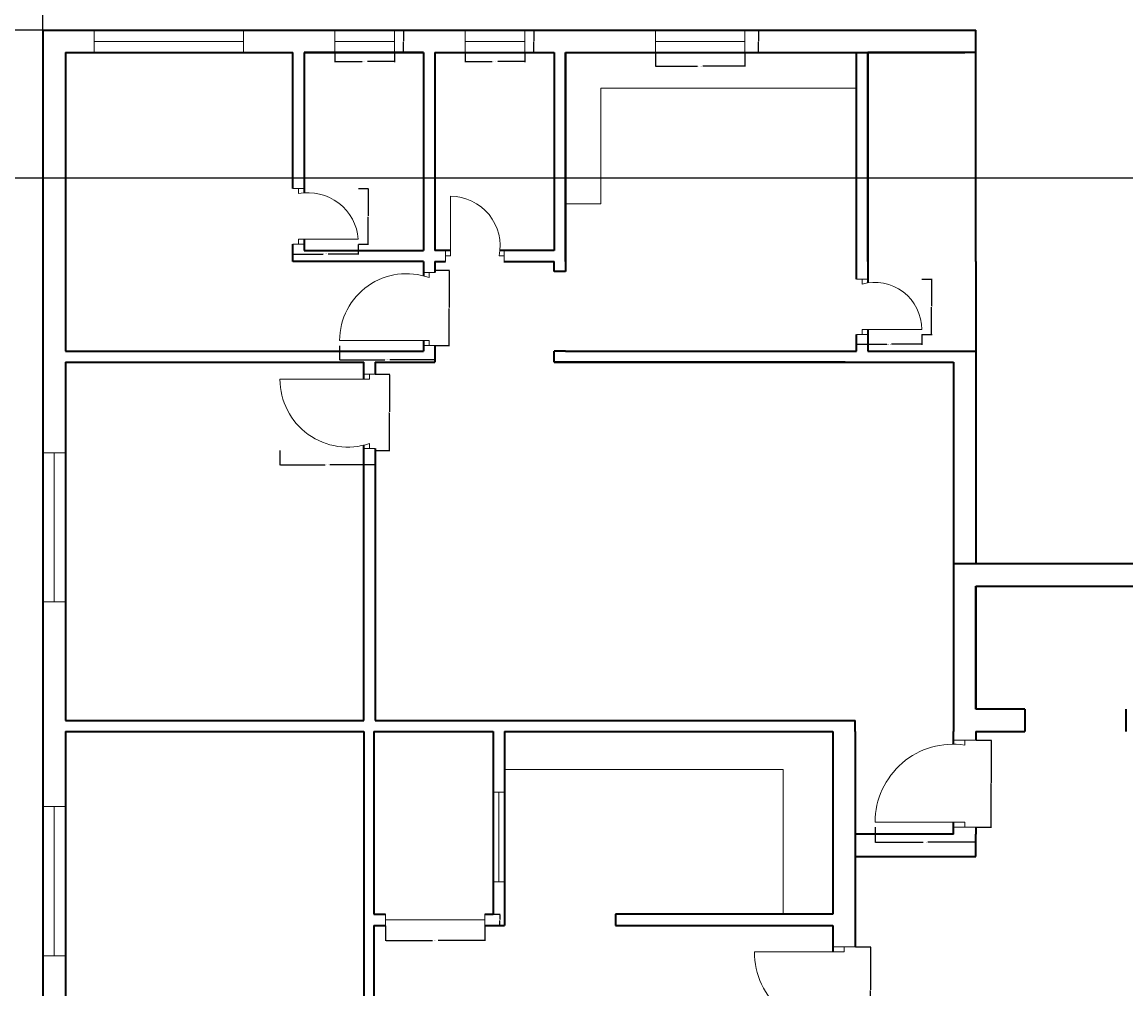
# Model space of a CAD drawing. Units: inches. Extents: x 2120 to 4013, y 1390 to 3019.
# Tile 52 of 59: x 3063 to 3507, y 1967 to 2356. Entities that reach past the tile are written whole.
import ezdxf

# ---------------------------------------------------------------- set-up
doc = ezdxf.new("R2010")
doc.units = ezdxf.units.IN
for name, color, linetype, lineweight in [('A-ANNO-DIMS', 2, 'Continuous', 18), ('A-ANNO-SYMB', 2, 'Continuous', 25), ('A-DOOR', 3, 'Continuous', 18), ('A-FLOR-CASE', 8, 'Continuous', 18), ('A-FURN', 8, 'Continuous', 13), ('A-GLAZ', 4, 'Continuous', 18), ('A-WALL', 7, 'Continuous', 35)]:
    doc.layers.add(name, color=color, linetype=linetype, lineweight=lineweight)
doc.styles.get("Standard").update_dxf_attribs({"font": 'arial.ttf'})
doc.dimstyles.get("Standard").update_dxf_attribs({"dimtxt": 0.18, "dimasz": 0.18, "dimexe": 0.18, "dimexo": 0.0625, "dimgap": 0.09, "dimtad": 0, "dimtih": 1, "dimtoh": 1, "dimdec": 4, "dimzin": 0, "dimdsep": 46, "dimtxsty": 'Standard', "dimcen": 0.09, "dimadec": 0, "dimazin": 0, "dimtfac": 1, "dimtdec": 4, "dimtofl": 0, "dimtmove": 0, "dimatfit": 3, "dimfxl": 1, "dimtolj": 1, "dimtzin": 0, "dimarcsym": 0})

# ---------------------------------------------------------------- blocks, each defined once
blk = doc.blocks.new('DOOR-SWING-24IN-96p73DEG')
for p, q in [((4.5, 22.36), (0, 22.36)), ((0, 22.36), (2.25, 22.36)), ((2.25, 22.36), (2.25, 20.36)), ((2.25, 0), (2.25, 2)), ((2.25, 2), (26.25, 2)), ((4.5, 0), (0, 0)), ((0, 0), (2.25, 0))]:
    blk.add_line(p, q)
blk.add_arc((6.09, 0.51), 20.22, 4.2154, 100.9483)
blk = doc.blocks.new('DOOR-SWING-24IN-101p88DEG')
for p, q in [((2, 2.25), (2, 26.25)), ((0, 4.5), (0, 0)), ((23.48, 4.5), (23.48, 0)), ((0, 0), (0, 2.25)), ((0, 2.25), (2, 2.25)), ((23.48, 2.25), (21.48, 2.25)), ((23.48, 0), (23.48, 2.25))]:
    blk.add_line(p, q)
blk.add_arc((2, 6.35), 19.9, 348.1217, 90)
blk = doc.blocks.new('DOOR-SWING-24IN-105p37DEG')
for p, q in [((4.5, 22.29), (0, 22.29)), ((0, 22.29), (2.25, 22.29)), ((2.25, 22.29), (2.25, 20.29)), ((0, 0), (4.5, 0)), ((2.25, 0), (2.25, 2)), ((2.25, 2), (26.25, 2)), ((4.5, 0), (2.25, 0))]:
    blk.add_line(p, q)
blk.add_arc((7.28, 2), 18.97, 0, 105.3718)
blk = doc.blocks.new('DOOR-SWING-36IN-109p78DEG')
for p, q in [((33.75, 29.31), (38.25, 29.31)), ((38.25, 29.31), (36, 29.31)), ((36, 29.31), (36, 27.31)), ((36, 2), (0, 2)), ((33.75, 0), (38.25, 0)), ((38.25, 0), (35.24, 0)), ((35.24, 0), (36, 0)), ((36, 0), (36, 2))]:
    blk.add_line(p, q)
blk.add_arc((26.9, 2), 26.9, 70.2228, 180)
blk = doc.blocks.new('DOOR-SWING-36IN-108p68DEG')
for p, q in [((36, 27.83), (0, 27.83)), ((38.25, 29.83), (33.75, 29.83)), ((33.75, 29.83), (36, 29.83)), ((36, 29.83), (36, 27.83)), ((36, 0), (36, 2)), ((33.75, 0), (38.25, 0)), ((38.25, 0), (36, 0))]:
    blk.add_line(p, q)
blk.add_arc((27.27, 27.83), 27.27, 180, 288.6764)
blk = doc.blocks.new('DOOR-SWING-36IN-98p95DEG')
for p, q in [((36, 32.77), (0, 32.77)), ((31.5, 34.77), (40.5, 34.77)), ((40.5, 34.77), (36, 34.77)), ((36, 34.77), (36, 32.77)), ((31.5, 0), (40.5, 0)), ((36, 0), (36, 2)), ((40.5, 0), (36, 0))]:
    blk.add_line(p, q)
blk.add_arc((31.15, 32.77), 31.15, 180, 278.9496)
blk = doc.blocks.new('DOOR-SWING-36IN-98p61DEG')
for p, q in [((40.5, 34.96), (31.5, 34.96)), ((31.5, 34.96), (36, 34.96)), ((36, 34.96), (36, 32.96)), ((36, 2), (0, 2)), ((31.5, 0), (40.5, 0)), ((36, 0), (36, 2)), ((40.5, 0), (36, 0))]:
    blk.add_line(p, q)
blk.add_arc((31.31, 2), 31.31, 81.386, 180)
blk = doc.blocks.new('WIN-PLAN-24IN')
for p, q in [((0, 0), (0, 9)), ((0, 9), (0, 4.5)), ((24, 4.5), (24, 9)), ((24, 9), (24, 0)), ((0, 4.5), (24, 4.5)), ((0, 0), (0, 0))]:
    blk.add_line(p, q)
blk = doc.blocks.new('WIN-PLAN-24IN-02')
for p, q in [((0, 0), (0, 9)), ((0, 9), (0, 4.5)), ((24, 4.5), (24, 9)), ((24, 9), (24, 0)), ((0, 4.5), (24, 4.5))]:
    blk.add_line(p, q)
blk = doc.blocks.new('WIN-PLAN-60IN')
for p, q in [((0, 9), (0, 0)), ((60, 4.5), (60, 9)), ((60, 9), (60, 0)), ((0, 0), (0, 4.5)), ((0, 4.5), (60, 4.5))]:
    blk.add_line(p, q)
blk = doc.blocks.new('WIN-PLAN-60IN-02')
for p, q in [((0, 0), (0, 9)), ((0, 9), (0, 4.5)), ((60, 4.5), (60, 9)), ((60, 9), (60, 0)), ((0, 4.5), (60, 4.5))]:
    blk.add_line(p, q)
blk = doc.blocks.new('WIN-PLAN-36IN')
for p, q in [((0, 0), (0, 9)), ((0, 9), (0, 4.5)), ((36, 4.5), (36, 9)), ((36, 9), (36, 0)), ((0, 4.5), (36, 4.5))]:
    blk.add_line(p, q)
blk = doc.blocks.new('WIN-PLAN-36IN-02')
for p, q in [((2.25, 36), (0, 36)), ((0, 36), (4.5, 36)), ((2.25, 0), (2.25, 36)), ((0, 0), (4.5, 0)), ((4.5, 0), (2.25, 0))]:
    blk.add_line(p, q)
blk = doc.blocks.new('WIN-PLAN-40IN')
for p, q in [((0, 4.5), (0, 0)), ((39.95, 4.5), (39.95, 0)), ((39.95, 2.25), (0, 2.25)), ((39.95, 0), (39.95, 2.25))]:
    blk.add_line(p, q)
blk = doc.blocks.new('*D113')
at = {"layer": 'A-ANNO-DIMS', "color": 0, "lineweight": -2, "transparency": 16777216}
for p, q in [((3172.23, 2266.43), (3172.23, 2262.37)), ((3198.48, 2266.43), (3198.48, 2262.37)), ((3172.41, 2262.55), (3184.37, 2262.55)), ((3198.3, 2262.55), (3186.35, 2262.55))]:
    blk.add_line(p, q, dxfattribs=at)
at = {"layer": 'A-ANNO-DIMS', "color": 0, "transparency": 16777216}
for points in [[(3172.41, 2262.58), (3172.41, 2262.52), (3172.23, 2262.55)], [(3198.3, 2262.58), (3198.3, 2262.52), (3198.48, 2262.55)]]:
    blk.add_solid(points, dxfattribs=at)
at = {"layer": 'Defpoints', "color": 0, "transparency": 16777216}
for p in [(3172.23, 2266.49), (3198.48, 2266.49), (3198.48, 2262.55)]:
    blk.add_point(p, dxfattribs=at)
at = {"layer": 'A-ANNO-DIMS', "color": 0, "transparency": 16777216, "insert": (3185.36, 2262.55), "char_height": 0.18, "attachment_point": 5}
blk.add_mtext('\\A1;SWING 26 TYP.', dxfattribs=at)
blk = doc.blocks.new('*D114')
at = {"layer": 'A-ANNO-DIMS', "color": 0, "lineweight": -2, "transparency": 16777216}
for p, q in [((3198.55, 2288.85), (3202.6, 2288.85)), ((3202.42, 2288.67), (3202.42, 2277.85)), ((3202.42, 2266.67), (3202.42, 2277.49)), ((3198.55, 2266.49), (3202.6, 2266.49))]:
    blk.add_line(p, q, dxfattribs=at)
at = {"layer": 'A-ANNO-DIMS', "color": 0, "transparency": 16777216}
for points in [[(3202.39, 2288.67), (3202.45, 2288.67), (3202.42, 2288.85)], [(3202.39, 2266.67), (3202.45, 2266.67), (3202.42, 2266.49)]]:
    blk.add_solid(points, dxfattribs=at)
at = {"layer": 'Defpoints', "color": 0, "transparency": 16777216}
for p in [(3198.48, 2288.85), (3202.42, 2288.85), (3198.48, 2266.49)]:
    blk.add_point(p, dxfattribs=at)
at = {"layer": 'A-ANNO-DIMS', "color": 0, "transparency": 16777216, "insert": (3202.42, 2277.67), "char_height": 0.18, "attachment_point": 5}
blk.add_mtext('\\A1;22 TYP.', dxfattribs=at)
blk = doc.blocks.new('*D117')
at = {"layer": 'A-ANNO-DIMS', "color": 0, "lineweight": -2, "transparency": 16777216}
for p, q in [((3398.73, 2230.14), (3398.73, 2226.08)), ((3424.98, 2230.14), (3424.98, 2226.08)), ((3398.91, 2226.26), (3410.87, 2226.26)), ((3424.8, 2226.26), (3412.85, 2226.26))]:
    blk.add_line(p, q, dxfattribs=at)
at = {"layer": 'A-ANNO-DIMS', "color": 0, "transparency": 16777216}
for points in [[(3398.91, 2226.29), (3398.91, 2226.23), (3398.73, 2226.26)], [(3424.8, 2226.29), (3424.8, 2226.23), (3424.98, 2226.26)]]:
    blk.add_solid(points, dxfattribs=at)
at = {"layer": 'Defpoints', "color": 0, "transparency": 16777216}
for p in [(3398.73, 2230.2), (3424.98, 2230.2), (3424.98, 2226.26)]:
    blk.add_point(p, dxfattribs=at)
at = {"layer": 'A-ANNO-DIMS', "color": 0, "transparency": 16777216, "insert": (3411.86, 2226.26), "char_height": 0.18, "attachment_point": 5}
blk.add_mtext('\\A1;SWING 26 TYP.', dxfattribs=at)
blk = doc.blocks.new('*D118')
at = {"layer": 'A-ANNO-DIMS', "color": 0, "lineweight": -2, "transparency": 16777216}
for p, q in [((3425.05, 2252.49), (3429.1, 2252.49)), ((3428.92, 2252.31), (3428.92, 2241.53)), ((3428.92, 2230.38), (3428.92, 2241.16)), ((3425.05, 2230.2), (3429.1, 2230.2))]:
    blk.add_line(p, q, dxfattribs=at)
at = {"layer": 'A-ANNO-DIMS', "color": 0, "transparency": 16777216}
for points in [[(3428.89, 2252.31), (3428.95, 2252.31), (3428.92, 2252.49)], [(3428.89, 2230.38), (3428.95, 2230.38), (3428.92, 2230.2)]]:
    blk.add_solid(points, dxfattribs=at)
at = {"layer": 'Defpoints', "color": 0, "transparency": 16777216}
for p in [(3424.98, 2252.49), (3428.92, 2252.49), (3424.98, 2230.2)]:
    blk.add_point(p, dxfattribs=at)
at = {"layer": 'A-ANNO-DIMS', "color": 0, "transparency": 16777216, "insert": (3428.92, 2241.35), "char_height": 0.18, "attachment_point": 5}
blk.add_mtext('\\A1;22 TYP.', dxfattribs=at)
blk = doc.blocks.new('*D143')
at = {"layer": 'A-ANNO-DIMS', "color": 0, "lineweight": -2, "transparency": 16777216}
for p, q in [((3190.98, 2225.69), (3190.98, 2219.84)), ((3229.23, 2225.69), (3229.23, 2219.84)), ((3191.16, 2220.02), (3209.12, 2220.02)), ((3229.05, 2220.02), (3211.1, 2220.02))]:
    blk.add_line(p, q, dxfattribs=at)
at = {"layer": 'A-ANNO-DIMS', "color": 0, "transparency": 16777216}
for points in [[(3191.16, 2220.05), (3191.16, 2219.99), (3190.98, 2220.02)], [(3229.05, 2220.05), (3229.05, 2219.99), (3229.23, 2220.02)]]:
    blk.add_solid(points, dxfattribs=at)
at = {"layer": 'Defpoints', "color": 0, "transparency": 16777216}
for p in [(3190.98, 2225.75), (3229.23, 2225.75), (3229.23, 2220.02)]:
    blk.add_point(p, dxfattribs=at)
at = {"layer": 'A-ANNO-DIMS', "color": 0, "transparency": 16777216, "insert": (3210.11, 2220.02), "char_height": 0.18, "attachment_point": 5}
blk.add_mtext('\\A1;SWING 38 TYP.', dxfattribs=at)
blk = doc.blocks.new('*D144')
at = {"layer": 'A-ANNO-DIMS', "color": 0, "lineweight": -2, "transparency": 16777216}
for p, q in [((3229.3, 2256.03), (3235.15, 2256.03)), ((3234.97, 2255.85), (3234.97, 2241.07)), ((3234.97, 2225.93), (3234.97, 2240.71)), ((3229.3, 2225.75), (3235.15, 2225.75))]:
    blk.add_line(p, q, dxfattribs=at)
at = {"layer": 'A-ANNO-DIMS', "color": 0, "transparency": 16777216}
for points in [[(3234.94, 2255.85), (3235, 2255.85), (3234.97, 2256.03)], [(3234.94, 2225.93), (3235, 2225.93), (3234.97, 2225.75)]]:
    blk.add_solid(points, dxfattribs=at)
at = {"layer": 'Defpoints', "color": 0, "transparency": 16777216}
for p in [(3229.23, 2256.03), (3234.97, 2256.03), (3229.23, 2225.75)]:
    blk.add_point(p, dxfattribs=at)
at = {"layer": 'A-ANNO-DIMS', "color": 0, "transparency": 16777216, "insert": (3234.97, 2240.89), "char_height": 0.18, "attachment_point": 5}
blk.add_mtext('\\A1;30 TYP.', dxfattribs=at)
blk = doc.blocks.new('*D145')
at = {"layer": 'A-ANNO-DIMS', "color": 0, "lineweight": -2, "transparency": 16777216}
for p, q in [((3166.98, 2183.48), (3166.98, 2177.63)), ((3205.23, 2183.48), (3205.23, 2177.63)), ((3167.16, 2177.81), (3185.12, 2177.81)), ((3205.05, 2177.81), (3187.1, 2177.81))]:
    blk.add_line(p, q, dxfattribs=at)
at = {"layer": 'A-ANNO-DIMS', "color": 0, "transparency": 16777216}
for points in [[(3167.16, 2177.84), (3167.16, 2177.78), (3166.98, 2177.81)], [(3205.05, 2177.84), (3205.05, 2177.78), (3205.23, 2177.81)]]:
    blk.add_solid(points, dxfattribs=at)
at = {"layer": 'Defpoints', "color": 0, "transparency": 16777216}
for p in [(3166.98, 2183.54), (3205.23, 2183.54), (3205.23, 2177.81)]:
    blk.add_point(p, dxfattribs=at)
at = {"layer": 'A-ANNO-DIMS', "color": 0, "transparency": 16777216, "insert": (3186.11, 2177.81), "char_height": 0.18, "attachment_point": 5}
blk.add_mtext('\\A1;SWING 38 TYP.', dxfattribs=at)
blk = doc.blocks.new('*D146')
at = {"layer": 'A-ANNO-DIMS', "color": 0, "lineweight": -2, "transparency": 16777216}
for p, q in [((3205.3, 2214.19), (3211.15, 2214.19)), ((3210.97, 2214.01), (3210.97, 2199.05)), ((3210.97, 2183.72), (3210.97, 2198.68)), ((3205.3, 2183.54), (3211.15, 2183.54))]:
    blk.add_line(p, q, dxfattribs=at)
at = {"layer": 'A-ANNO-DIMS', "color": 0, "transparency": 16777216}
for points in [[(3210.94, 2214.01), (3211, 2214.01), (3210.97, 2214.19)], [(3210.94, 2183.72), (3211, 2183.72), (3210.97, 2183.54)]]:
    blk.add_solid(points, dxfattribs=at)
at = {"layer": 'Defpoints', "color": 0, "transparency": 16777216}
for p in [(3205.23, 2214.19), (3210.97, 2214.19), (3205.23, 2183.54)]:
    blk.add_point(p, dxfattribs=at)
at = {"layer": 'A-ANNO-DIMS', "color": 0, "transparency": 16777216, "insert": (3210.97, 2198.87), "char_height": 0.18, "attachment_point": 5}
blk.add_mtext('\\A1;31 TYP.', dxfattribs=at)
blk = doc.blocks.new('*D150')
at = {"layer": 'A-ANNO-DIMS', "color": 0, "lineweight": -2, "transparency": 16777216}
for p, q in [((3398.3, 1983.94), (3404.49, 1983.94)), ((3404.31, 1983.76), (3404.31, 1966.73)), ((3404.31, 1949.34), (3404.31, 1966.37)), ((3398.3, 1949.16), (3404.49, 1949.16))]:
    blk.add_line(p, q, dxfattribs=at)
at = {"layer": 'A-ANNO-DIMS', "color": 0, "transparency": 16777216}
for points in [[(3404.28, 1983.76), (3404.34, 1983.76), (3404.31, 1983.94)], [(3404.28, 1949.34), (3404.34, 1949.34), (3404.31, 1949.16)]]:
    blk.add_solid(points, dxfattribs=at)
at = {"layer": 'Defpoints', "color": 0, "transparency": 16777216}
for p in [(3398.23, 1983.94), (3404.31, 1983.94), (3398.23, 1949.16)]:
    blk.add_point(p, dxfattribs=at)
at = {"layer": 'A-ANNO-DIMS', "color": 0, "transparency": 16777216, "insert": (3404.31, 1966.55), "char_height": 0.18, "attachment_point": 5}
blk.add_mtext('\\A1;35 TYP.', dxfattribs=at)
blk = doc.blocks.new('*D155')
at = {"layer": 'A-ANNO-DIMS', "color": 0, "lineweight": -2, "transparency": 16777216}
for p, q in [((3406.23, 2032.08), (3406.23, 2025.89)), ((3446.73, 2032.08), (3446.73, 2025.89)), ((3406.41, 2026.07), (3425.5, 2026.07)), ((3446.55, 2026.07), (3427.47, 2026.07))]:
    blk.add_line(p, q, dxfattribs=at)
at = {"layer": 'A-ANNO-DIMS', "color": 0, "transparency": 16777216}
for points in [[(3406.41, 2026.1), (3406.41, 2026.04), (3406.23, 2026.07)], [(3446.55, 2026.1), (3446.55, 2026.04), (3446.73, 2026.07)]]:
    blk.add_solid(points, dxfattribs=at)
at = {"layer": 'Defpoints', "color": 0, "transparency": 16777216}
for p in [(3406.23, 2032.14), (3446.73, 2032.14), (3446.73, 2026.07)]:
    blk.add_point(p, dxfattribs=at)
at = {"layer": 'A-ANNO-DIMS', "color": 0, "transparency": 16777216, "insert": (3426.48, 2026.07), "char_height": 0.18, "attachment_point": 5}
blk.add_mtext('\\A1;SWING 41 TYP.', dxfattribs=at)
blk = doc.blocks.new('*D156')
at = {"layer": 'A-ANNO-DIMS', "color": 0, "lineweight": -2, "transparency": 16777216}
for p, q in [((3446.8, 2067.1), (3452.99, 2067.1)), ((3452.81, 2066.92), (3452.81, 2049.8)), ((3452.81, 2032.32), (3452.81, 2049.44)), ((3446.8, 2032.14), (3452.99, 2032.14))]:
    blk.add_line(p, q, dxfattribs=at)
at = {"layer": 'A-ANNO-DIMS', "color": 0, "transparency": 16777216}
for points in [[(3452.78, 2066.92), (3452.84, 2066.92), (3452.81, 2067.1)], [(3452.78, 2032.32), (3452.84, 2032.32), (3452.81, 2032.14)]]:
    blk.add_solid(points, dxfattribs=at)
at = {"layer": 'Defpoints', "color": 0, "transparency": 16777216}
for p in [(3446.73, 2067.1), (3452.81, 2067.1), (3446.73, 2032.14)]:
    blk.add_point(p, dxfattribs=at)
at = {"layer": 'A-ANNO-DIMS', "color": 0, "transparency": 16777216, "insert": (3452.81, 2049.62), "char_height": 0.18, "attachment_point": 5}
blk.add_mtext('\\A1;35 TYP.', dxfattribs=at)
blk = doc.blocks.new('*D175')
at = {"layer": 'A-ANNO-DIMS', "color": 0, "lineweight": -2, "transparency": 16777216}
for p, q in [((3241.44, 2343.47), (3241.44, 2339.75)), ((3265.44, 2343.47), (3265.44, 2339.75)), ((3241.62, 2339.93), (3252.32, 2339.93)), ((3265.26, 2339.93), (3254.55, 2339.93))]:
    blk.add_line(p, q, dxfattribs=at)
at = {"layer": 'A-ANNO-DIMS', "color": 0, "transparency": 16777216}
for points in [[(3241.62, 2339.96), (3241.62, 2339.9), (3241.44, 2339.93)], [(3265.26, 2339.96), (3265.26, 2339.9), (3265.44, 2339.93)]]:
    blk.add_solid(points, dxfattribs=at)
at = {"layer": 'Defpoints', "color": 0, "transparency": 16777216}
for p in [(3241.44, 2343.53), (3265.44, 2343.53), (3265.44, 2339.93)]:
    blk.add_point(p, dxfattribs=at)
at = {"layer": 'A-ANNO-DIMS', "color": 0, "transparency": 16777216, "insert": (3253.44, 2339.93), "char_height": 0.18, "attachment_point": 5}
blk.add_mtext('\\A1;WINDOW 24 TYP.', dxfattribs=at)
blk = doc.blocks.new('*D176')
at = {"layer": 'A-ANNO-DIMS', "color": 0, "lineweight": -2, "transparency": 16777216}
for p, q in [((3265.5, 2352.53), (3269.22, 2352.53)), ((3269.04, 2352.35), (3269.04, 2348.21)), ((3269.04, 2343.71), (3269.04, 2347.85)), ((3265.5, 2343.53), (3269.22, 2343.53))]:
    blk.add_line(p, q, dxfattribs=at)
at = {"layer": 'A-ANNO-DIMS', "color": 0, "transparency": 16777216}
for points in [[(3269.01, 2352.35), (3269.07, 2352.35), (3269.04, 2352.53)], [(3269.01, 2343.71), (3269.07, 2343.71), (3269.04, 2343.53)]]:
    blk.add_solid(points, dxfattribs=at)
at = {"layer": 'Defpoints', "color": 0, "transparency": 16777216}
for p in [(3265.44, 2352.53), (3269.04, 2352.53), (3265.44, 2343.53)]:
    blk.add_point(p, dxfattribs=at)
at = {"layer": 'A-ANNO-DIMS', "color": 0, "transparency": 16777216, "insert": (3269.04, 2348.03), "char_height": 0.18, "attachment_point": 5}
blk.add_mtext('\\A1;9 TYP.', dxfattribs=at)
blk = doc.blocks.new('*D177')
at = {"layer": 'A-ANNO-DIMS', "color": 0, "lineweight": -2, "transparency": 16777216}
for p, q in [((3317.91, 2343.47), (3317.91, 2337.95)), ((3353.91, 2343.47), (3353.91, 2337.95)), ((3318.09, 2338.13), (3334.79, 2338.13)), ((3353.73, 2338.13), (3337.03, 2338.13))]:
    blk.add_line(p, q, dxfattribs=at)
at = {"layer": 'A-ANNO-DIMS', "color": 0, "transparency": 16777216}
for points in [[(3318.09, 2338.16), (3318.09, 2338.1), (3317.91, 2338.13)], [(3353.73, 2338.16), (3353.73, 2338.1), (3353.91, 2338.13)]]:
    blk.add_solid(points, dxfattribs=at)
at = {"layer": 'Defpoints', "color": 0, "transparency": 16777216}
for p in [(3317.91, 2343.53), (3353.91, 2343.53), (3353.91, 2338.13)]:
    blk.add_point(p, dxfattribs=at)
at = {"layer": 'A-ANNO-DIMS', "color": 0, "transparency": 16777216, "insert": (3335.91, 2338.13), "char_height": 0.18, "attachment_point": 5}
blk.add_mtext('\\A1;WINDOW 36 TYP.', dxfattribs=at)
blk = doc.blocks.new('*D178')
at = {"layer": 'A-ANNO-DIMS', "color": 0, "lineweight": -2, "transparency": 16777216}
for p, q in [((3353.98, 2352.53), (3359.49, 2352.53)), ((3359.31, 2352.35), (3359.31, 2348.21)), ((3359.31, 2343.71), (3359.31, 2347.85)), ((3353.98, 2343.53), (3359.49, 2343.53))]:
    blk.add_line(p, q, dxfattribs=at)
at = {"layer": 'A-ANNO-DIMS', "color": 0, "transparency": 16777216}
for points in [[(3359.28, 2352.35), (3359.34, 2352.35), (3359.31, 2352.53)], [(3359.28, 2343.71), (3359.34, 2343.71), (3359.31, 2343.53)]]:
    blk.add_solid(points, dxfattribs=at)
at = {"layer": 'Defpoints', "color": 0, "transparency": 16777216}
for p in [(3353.91, 2352.53), (3359.31, 2352.53), (3353.91, 2343.53)]:
    blk.add_point(p, dxfattribs=at)
at = {"layer": 'A-ANNO-DIMS', "color": 0, "transparency": 16777216, "insert": (3359.31, 2348.03), "char_height": 0.18, "attachment_point": 5}
blk.add_mtext('\\A1;9 TYP.', dxfattribs=at)
blk = doc.blocks.new('*D181')
at = {"layer": 'A-ANNO-DIMS', "color": 0, "lineweight": -2, "transparency": 16777216}
for p, q in [((3189.1, 2343.47), (3189.1, 2339.75)), ((3213.1, 2343.47), (3213.1, 2339.75)), ((3189.28, 2339.93), (3199.98, 2339.93)), ((3212.92, 2339.93), (3202.21, 2339.93))]:
    blk.add_line(p, q, dxfattribs=at)
at = {"layer": 'A-ANNO-DIMS', "color": 0, "transparency": 16777216}
for points in [[(3189.28, 2339.96), (3189.28, 2339.9), (3189.1, 2339.93)], [(3212.92, 2339.96), (3212.92, 2339.9), (3213.1, 2339.93)]]:
    blk.add_solid(points, dxfattribs=at)
at = {"layer": 'Defpoints', "color": 0, "transparency": 16777216}
for p in [(3189.1, 2343.53), (3213.1, 2343.53), (3213.1, 2339.93)]:
    blk.add_point(p, dxfattribs=at)
at = {"layer": 'A-ANNO-DIMS', "color": 0, "transparency": 16777216, "insert": (3201.1, 2339.93), "char_height": 0.18, "attachment_point": 5}
blk.add_mtext('\\A1;WINDOW 24 TYP.', dxfattribs=at)
blk = doc.blocks.new('*D182')
at = {"layer": 'A-ANNO-DIMS', "color": 0, "lineweight": -2, "transparency": 16777216}
for p, q in [((3213.16, 2352.53), (3216.88, 2352.53)), ((3216.7, 2352.35), (3216.7, 2348.21)), ((3216.7, 2343.71), (3216.7, 2347.85)), ((3213.16, 2343.53), (3216.88, 2343.53))]:
    blk.add_line(p, q, dxfattribs=at)
at = {"layer": 'A-ANNO-DIMS', "color": 0, "transparency": 16777216}
for points in [[(3216.67, 2352.35), (3216.73, 2352.35), (3216.7, 2352.53)], [(3216.67, 2343.71), (3216.73, 2343.71), (3216.7, 2343.53)]]:
    blk.add_solid(points, dxfattribs=at)
at = {"layer": 'Defpoints', "color": 0, "transparency": 16777216}
for p in [(3213.1, 2352.53), (3216.7, 2352.53), (3213.1, 2343.53)]:
    blk.add_point(p, dxfattribs=at)
at = {"layer": 'A-ANNO-DIMS', "color": 0, "transparency": 16777216, "insert": (3216.7, 2348.03), "char_height": 0.18, "attachment_point": 5}
blk.add_mtext('\\A1;9 TYP.', dxfattribs=at)
blk = doc.blocks.new('*D195')
at = {"layer": 'A-ANNO-DIMS', "color": 0, "lineweight": -2, "transparency": 16777216}
for p, q in [((3209.45, 1992.47), (3209.45, 1986.36)), ((3249.4, 1992.47), (3249.4, 1986.36)), ((3209.63, 1986.54), (3228.31, 1986.54)), ((3249.22, 1986.54), (3230.54, 1986.54))]:
    blk.add_line(p, q, dxfattribs=at)
at = {"layer": 'A-ANNO-DIMS', "color": 0, "transparency": 16777216}
for points in [[(3209.63, 1986.57), (3209.63, 1986.51), (3209.45, 1986.54)], [(3249.22, 1986.57), (3249.22, 1986.51), (3249.4, 1986.54)]]:
    blk.add_solid(points, dxfattribs=at)
at = {"layer": 'Defpoints', "color": 0, "transparency": 16777216}
for p in [(3209.45, 1992.53), (3249.4, 1992.53), (3249.4, 1986.54)]:
    blk.add_point(p, dxfattribs=at)
at = {"layer": 'A-ANNO-DIMS', "color": 0, "transparency": 16777216, "insert": (3229.43, 1986.54), "char_height": 0.18, "attachment_point": 5}
blk.add_mtext('\\A1;WINDOW 40 TYP.', dxfattribs=at)
blk = doc.blocks.new('*D196')
at = {"layer": 'A-ANNO-DIMS', "color": 0, "lineweight": -2, "transparency": 16777216}
for p, q in [((3249.46, 1997.03), (3255.57, 1997.03)), ((3255.39, 1996.85), (3255.39, 1994.96)), ((3249.46, 1992.53), (3255.57, 1992.53)), ((3255.39, 1992.71), (3255.39, 1994.6))]:
    blk.add_line(p, q, dxfattribs=at)
at = {"layer": 'A-ANNO-DIMS', "color": 0, "transparency": 16777216}
for points in [[(3255.36, 1996.85), (3255.42, 1996.85), (3255.39, 1997.03)], [(3255.36, 1992.71), (3255.42, 1992.71), (3255.39, 1992.53)]]:
    blk.add_solid(points, dxfattribs=at)
at = {"layer": 'Defpoints', "color": 0, "transparency": 16777216}
for p in [(3249.4, 1997.03), (3255.39, 1997.03), (3249.4, 1992.53)]:
    blk.add_point(p, dxfattribs=at)
at = {"layer": 'A-ANNO-DIMS', "color": 0, "transparency": 16777216, "insert": (3255.39, 1994.78), "char_height": 0.18, "attachment_point": 5}
blk.add_mtext('\\A1;5 TYP.', dxfattribs=at)
blk = doc.blocks.new('*D216')
at = {"layer": 'A-ANNO-DIMS', "color": 0, "lineweight": -2, "transparency": 16777216}
for p, q in [((3071.73, 2352.59), (3071.73, 2396.46)), ((3071.91, 2396.28), (3444.95, 2396.28)), ((3818.55, 2396.28), (3445.52, 2396.28)), ((3818.73, 2352.59), (3818.73, 2396.46))]:
    blk.add_line(p, q, dxfattribs=at)
at = {"layer": 'A-ANNO-DIMS', "color": 0, "transparency": 16777216}
for points in [[(3071.91, 2396.31), (3071.91, 2396.25), (3071.73, 2396.28)], [(3818.55, 2396.31), (3818.55, 2396.25), (3818.73, 2396.28)]]:
    blk.add_solid(points, dxfattribs=at)
at = {"layer": 'Defpoints', "color": 0, "transparency": 16777216}
for p in [(3818.73, 2396.28), (3071.73, 2352.53), (3818.73, 2352.53)]:
    blk.add_point(p, dxfattribs=at)
at = {"layer": 'A-ANNO-DIMS', "color": 0, "transparency": 16777216, "insert": (3445.23, 2396.28), "char_height": 0.18, "attachment_point": 5}
blk.add_mtext('\\A1;747', dxfattribs=at)
blk = doc.blocks.new('*D217')
at = {"layer": 'A-ANNO-DIMS', "color": 0, "lineweight": -2, "transparency": 16777216}
for p, q in [((3071.67, 2352.53), (2980.31, 2352.53)), ((2980.49, 2352.35), (2980.49, 1947.71)), ((2980.49, 1542.71), (2980.49, 1947.35)), ((3305.67, 1542.53), (2980.31, 1542.53))]:
    blk.add_line(p, q, dxfattribs=at)
at = {"layer": 'A-ANNO-DIMS', "color": 0, "transparency": 16777216}
for points in [[(2980.46, 2352.35), (2980.52, 2352.35), (2980.49, 2352.53)], [(2980.46, 1542.71), (2980.52, 1542.71), (2980.49, 1542.53)]]:
    blk.add_solid(points, dxfattribs=at)
at = {"layer": 'Defpoints', "color": 0, "transparency": 16777216}
for p in [(2980.49, 2352.53), (3071.73, 2352.53), (3305.73, 1542.53)]:
    blk.add_point(p, dxfattribs=at)
at = {"layer": 'A-ANNO-DIMS', "color": 0, "transparency": 16777216, "insert": (2980.49, 1947.53), "char_height": 0.18, "attachment_point": 5}
blk.add_mtext('\\A1;810', dxfattribs=at)

msp = doc.modelspace()

# ---------------------------------------------------------------- linework, layer by layer
at = {"layer": 'A-ANNO-SYMB'}
msp.add_line((3024.2377, 2293.2324), (3883.8033, 2293.2324), dxfattribs=at)
at = {"layer": 'A-FLOR-CASE'}
for p, q in [((3295.9316, 2282.7615), (3295.9316, 2329.2074)), ((3295.9316, 2329.2074), (3398.7347, 2329.2074)), ((3281.7347, 2282.7615), (3295.9316, 2282.7615)), ((3257.2347, 2055.3306), (3369.3205, 2055.3306)), ((3369.3205, 2055.3306), (3369.3205, 1997.031))]:
    msp.add_line(p, q, dxfattribs=at)
at = {"layer": 'A-FURN'}
for p, q in [((3096.1722, 2343.531), (3143.9625, 2343.531)), ((3080.7347, 2117.0577), (3080.7347, 2164.848)), ((3080.7347, 1997.0953), (3080.7347, 2044.8856))]:
    msp.add_line(p, q, dxfattribs=at)
at = {"layer": 'A-WALL'}
for p, q in [((3071.7347, 2352.531), (3446.7347, 2352.531)), ((3071.7347, 2352.531), (3071.7347, 1581.531)), ((3446.7347, 2259.531), (3446.7347, 2352.531)), ((3080.7347, 2343.531), (3172.2347, 2343.531)), ((3080.7347, 2343.531), (3080.7347, 2223.531)), ((3172.2347, 2288.8489), (3172.2347, 2343.531)), ((3176.7347, 2343.531), (3224.7347, 2343.531)), ((3224.7347, 2343.531), (3176.7347, 2343.531)), ((3176.7347, 2343.531), (3176.7347, 2287.1543)), ((3224.7347, 2343.531), (3224.7347, 2264.031)), ((3229.2347, 2343.531), (3277.2347, 2343.531)), ((3229.2347, 2343.531), (3229.2347, 2264.031)), ((3229.2347, 2343.531), (3277.2347, 2343.531)), ((3277.2347, 2343.531), (3277.2347, 2264.031)), ((3281.7347, 2343.531), (3398.7347, 2343.531)), ((3281.7347, 2259.531), (3281.7347, 2343.531)), ((3281.7347, 2343.531), (3281.7347, 2255.5496)), ((3394.2347, 2343.531), (3442.2347, 2343.531)), ((3398.7347, 2259.531), (3398.7347, 2343.531)), ((3403.2347, 2259.531), (3403.2347, 2343.531)), ((3446.7347, 2343.531), (3403.2347, 2343.531)), ((3403.2347, 2343.531), (3403.2347, 2250.9655)), ((3176.7347, 2268.4875), (3176.7347, 2264.031)), ((3172.2347, 2259.531), (3172.2347, 2266.4875)), ((3176.7347, 2264.031), (3224.7347, 2264.031)), ((3235.5732, 2264.031), (3229.2347, 2264.031)), ((3277.2347, 2264.031), (3255.3906, 2264.031)), ((3398.7347, 2252.4915), (3398.7347, 2263.191)), ((3176.7347, 2259.531), (3172.2347, 2259.531)), ((3224.7347, 2259.531), (3176.7347, 2259.531)), ((3224.7347, 2259.531), (3224.7347, 2253.7651)), ((3229.2347, 2259.531), (3229.2347, 2255.0658)), ((3229.2347, 2259.531), (3233.5732, 2259.531)), ((3257.0503, 2259.531), (3277.2347, 2259.531)), ((3277.2347, 2255.5496), (3277.2347, 2259.531)), ((3403.2347, 2259.531), (3403.2347, 2250.9655)), ((3446.7347, 2259.531), (3446.7347, 2138.031)), ((3281.7347, 2255.5496), (3277.2347, 2255.5496)), ((3403.2347, 2232.1991), (3403.2347, 2223.531)), ((3403.2347, 2232.1991), (3403.2347, 2223.531)), ((3224.7347, 2227.7538), (3224.7347, 2223.531)), ((3398.7347, 2223.531), (3398.7347, 2230.1991)), ((3080.7347, 2223.531), (3224.7347, 2223.531)), ((3200.7347, 2223.531), (3205.2347, 2223.531)), ((3229.2347, 2225.7538), (3229.2347, 2219.031)), ((3277.2347, 2219.031), (3277.2347, 2223.531)), ((3281.7347, 2223.531), (3277.2347, 2223.531)), ((3281.7347, 2223.531), (3398.7347, 2223.531)), ((3394.2347, 2223.531), (3398.7347, 2223.531)), ((3403.2347, 2223.531), (3446.7347, 2223.531)), ((3080.7347, 2219.031), (3200.7347, 2219.031)), ((3080.7347, 2219.031), (3080.7347, 2075.031)), ((3200.7347, 2212.189), (3200.7347, 2219.031)), ((3205.2347, 2219.031), (3229.2347, 2219.031)), ((3205.2347, 2219.031), (3205.2347, 2214.189)), ((3281.7347, 2219.031), (3277.2347, 2219.031)), ((3277.2347, 2219.031), (3437.7347, 2219.031)), ((3394.2347, 2219.031), (3281.7347, 2219.031)), ((3437.7347, 2219.031), (3437.7347, 2138.031)), ((3200.7347, 2075.031), (3200.7347, 2185.7025)), ((3205.2347, 2184.3568), (3205.2347, 2075.031)), ((3437.7347, 2138.031), (3437.7347, 2070.531)), ((3437.7347, 2138.031), (3437.7347, 2070.531)), ((3533.7347, 2138.031), (3437.7347, 2138.031)), ((3446.7347, 2129.031), (3446.7347, 2079.531)), ((3446.7347, 2079.531), (3446.7347, 2129.031)), ((3446.7347, 2129.031), (3524.7347, 2129.031)), ((3466.3428, 2079.531), (3446.7347, 2079.531)), ((3466.3428, 2079.531), (3466.3428, 2070.531)), ((3507.0394, 2079.531), (3507.0394, 2070.531)), ((3080.7347, 2075.031), (3200.7347, 2075.031)), ((3080.7347, 2075.031), (3200.7347, 2075.031)), ((3205.2347, 2075.031), (3398.2347, 2075.031)), ((3398.2347, 2070.531), (3398.2347, 2075.031)), ((3080.7347, 2070.531), (3200.7347, 2070.531)), ((3080.7347, 2070.531), (3080.7347, 1926.531)), ((3200.7347, 2070.531), (3200.7347, 1926.531)), ((3204.7347, 2070.531), (3252.7347, 2070.531)), ((3204.7347, 2070.531), (3204.7347, 1997.031)), ((3252.7347, 2070.531), (3252.7347, 1997.031)), ((3257.2347, 2070.531), (3389.2347, 2070.531)), ((3257.2347, 2070.531), (3257.2347, 1992.531)), ((3389.2347, 2070.531), (3389.2347, 1997.031)), ((3389.2347, 2070.531), (3389.2347, 1997.031)), ((3398.2347, 2070.531), (3398.2347, 1983.9368)), ((3437.7347, 2065.4513), (3437.7347, 2070.531)), ((3446.7347, 2070.531), (3466.3428, 2070.531)), ((3446.7347, 2070.531), (3446.7347, 2067.0987)), ((3437.7347, 2029.2261), (3437.7347, 2034.1415)), ((3437.7347, 2029.2261), (3398.2347, 2029.2261)), ((3446.7347, 2032.1415), (3446.7347, 2029.2261)), ((3446.7347, 2020.2261), (3446.7347, 2029.2261)), ((3398.2347, 2020.2261), (3446.7347, 2020.2261)), ((3204.7347, 1997.031), (3209.4526, 1997.031)), ((3249.3984, 1997.031), (3252.7347, 1997.031)), ((3389.2347, 1997.031), (3301.9091, 1997.031)), ((3301.9091, 1997.031), (3301.9091, 1992.531)), ((3204.7347, 1992.531), (3209.4526, 1992.531)), ((3204.7347, 1992.531), (3204.7347, 1922.531)), ((3249.3984, 1992.531), (3257.2347, 1992.531)), ((3301.9091, 1992.531), (3389.2347, 1992.531)), ((3389.2347, 1992.531), (3389.2347, 1981.9368))]:
    msp.add_line(p, q, dxfattribs=at)

# ---------------------------------------------------------------- block references
at = {"layer": 'A-DOOR'}
for name, p in [('DOOR-SWING-24IN-96p73DEG', (3172.2347, 2266.4875)), ('DOOR-SWING-24IN-101p88DEG', (3233.5732, 2259.531)), ('DOOR-SWING-36IN-109p78DEG', (3190.9847, 2225.7538)), ('DOOR-SWING-24IN-105p37DEG', (3398.7347, 2230.1991)), ('DOOR-SWING-36IN-108p68DEG', (3166.9847, 2184.3568)), ('DOOR-SWING-36IN-98p61DEG', (3406.2347, 2032.1415)), ('DOOR-SWING-36IN-98p95DEG', (3357.7347, 1949.1625))]:
    msp.add_blockref(name, p, dxfattribs=at)
at = {"layer": 'A-GLAZ'}
for name, p in [('WIN-PLAN-60IN', (3092.3803, 2343.531)), ('WIN-PLAN-24IN', (3189.0958, 2343.531)), ('WIN-PLAN-24IN-02', (3241.4354, 2343.531)), ('WIN-PLAN-36IN', (3317.9131, 2343.531)), ('WIN-PLAN-40IN', (3209.4526, 1992.531))]:
    msp.add_blockref(name, p, dxfattribs=at)
for name, p, rotation in [('WIN-PLAN-60IN', (3071.7347, 2182.638), 269.9999999999974), ('WIN-PLAN-36IN-02', (3257.2347, 2046.1368), 180), ('WIN-PLAN-60IN-02', (3080.7347, 1980.3893), 89.99999999999909)]:
    msp.add_blockref(name, p, dxfattribs=dict(at, rotation=rotation))

# ---------------------------------------------------------------- dimensions: what is measured, and where the dimension line sits
at = {"layer": 'A-ANNO-DIMS'}
dim = msp.add_linear_dim(base=(3818.7347, 2396.281), p1=(3071.7347, 2352.531), p2=(3818.7347, 2352.531), dimstyle='Standard', override={"dimdec": 0, "dimlfac": 1, "dimrnd": 0, "dimzin": 0, "dimdsep": 46, "dimlunit": 2}, dxfattribs=at)
dim.commit()
dim.dimension.update_dxf_attribs({"geometry": '*D216', "text_midpoint": (3445.2347, 2396.281)})
dim = msp.add_linear_dim(base=(2980.4877, 2352.531), p1=(3305.7347, 1542.531), p2=(3071.7347, 2352.531), angle=90, dimstyle='Standard', override={"dimdec": 0, "dimlfac": 1, "dimrnd": 0, "dimzin": 0, "dimdsep": 46, "dimlunit": 2}, dxfattribs=at)
dim.commit()
dim.dimension.update_dxf_attribs({"geometry": '*D217', "text_midpoint": (2980.4877, 1947.531)})
for base, p1, p2, picture, middle in [((3216.6958, 2352.531), (3213.0958, 2343.531), (3213.0958, 2352.531), '*D182', (3216.6958, 2348.031)), ((3269.0354, 2352.531), (3265.4354, 2343.531), (3265.4354, 2352.531), '*D176', (3269.0354, 2348.031)), ((3359.3131, 2352.531), (3353.9131, 2343.531), (3353.9131, 2352.531), '*D178', (3359.3131, 2348.031)), ((3202.4222, 2288.8489), (3198.4847, 2266.4875), (3198.4847, 2288.8489), '*D114', (3202.4222, 2277.6682)), ((3234.9722, 2256.029), (3229.2347, 2225.7538), (3229.2347, 2256.029), '*D144', (3234.9722, 2240.8914)), ((3428.9222, 2252.4915), (3424.9847, 2230.1991), (3424.9847, 2252.4915), '*D118', (3428.9222, 2241.3453)), ((3210.9722, 2214.189), (3205.2347, 2183.5435), (3205.2347, 2214.189), '*D146', (3210.9722, 2198.8662)), ((3452.8097, 2067.0987), (3446.7347, 2032.1415), (3446.7347, 2067.0987), '*D156', (3452.8097, 2049.6201)), ((3255.3902626884, 1997.03095126), (3249.398397414, 1992.53095126), (3249.398397414, 1997.03095126), '*D196', (3255.3902626884, 1994.78095126)), ((3404.3097, 1983.9368), (3398.2347, 1949.1625), (3398.2347, 1983.9368), '*D150', (3404.3097, 1966.5497))]:
    dim = msp.add_linear_dim(base=base, p1=p1, p2=p2, angle=90, text='<> TYP.', dimstyle='Standard', override={"dimdec": 0, "dimlfac": 1, "dimrnd": 0, "dimzin": 0, "dimdsep": 46, "dimlunit": 2}, dxfattribs=at)
    dim.commit()
    dim.dimension.update_dxf_attribs({"geometry": picture, "text_midpoint": middle})
for base, p1, p2, text, picture, middle in [((3213.0958, 2339.931), (3189.0958, 2343.531), (3213.0958, 2343.531), 'WINDOW <> TYP.', '*D181', (3201.0958, 2339.931)), ((3265.4354, 2339.931), (3241.4354, 2343.531), (3265.4354, 2343.531), 'WINDOW <> TYP.', '*D175', (3253.4354, 2339.931)), ((3353.9131, 2338.131), (3317.9131, 2343.531), (3353.9131, 2343.531), 'WINDOW <> TYP.', '*D177', (3335.9131, 2338.131)), ((3198.4847, 2262.55), (3172.2347, 2266.4875), (3198.4847, 2266.4875), 'SWING <> TYP.', '*D113', (3185.3597, 2262.55)), ((3424.9847, 2226.2616), (3398.7347, 2230.1991), (3424.9847, 2230.1991), 'SWING <> TYP.', '*D117', (3411.8597, 2226.2616)), ((3229.2347, 2220.0163), (3190.9847, 2225.7538), (3229.2347, 2225.7538), 'SWING <> TYP.', '*D143', (3210.1097, 2220.0163)), ((3205.2347, 2177.806), (3166.9847, 2183.5435), (3205.2347, 2183.5435), 'SWING <> TYP.', '*D145', (3186.1097, 2177.806)), ((3446.7346645849, 2026.066459598), (3406.2346645849, 2032.141459598), (3446.7346645849, 2032.141459598), 'SWING <> TYP.', '*D155', (3426.4846645849, 2026.066459598)), ((3249.3984, 1986.5391), (3209.4526, 1992.531), (3249.3984, 1992.531), 'WINDOW <> TYP.', '*D195', (3229.4255, 1986.5391))]:
    dim = msp.add_linear_dim(base=base, p1=p1, p2=p2, text=text, dimstyle='Standard', override={"dimdec": 0, "dimlfac": 1, "dimrnd": 0, "dimzin": 0, "dimdsep": 46, "dimlunit": 2}, dxfattribs=at)
    dim.commit()
    dim.dimension.update_dxf_attribs({"geometry": picture, "text_midpoint": middle})

doc.saveas('drawing.dxf')
